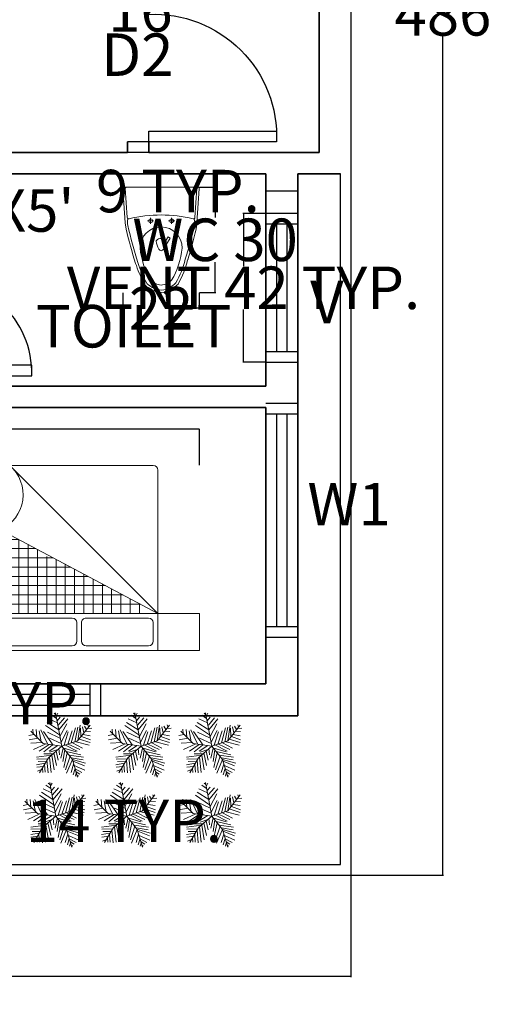
# Model space of a CAD drawing. Units: inches. Extents: x 774 to 1314, y 374 to 930.
# Tile 3 of 5: x 1137 to 1270, y 374 to 652. Entities that reach past the tile are written whole.
import ezdxf
from ezdxf.enums import TextEntityAlignment as Align

# ---------------------------------------------------------------- set-up
doc = ezdxf.new("R2010")
doc.units = ezdxf.units.IN
doc.header["$MEASUREMENT"] = 0
for name, color, linetype, lineweight in [('A-ANNO-DIMS', 2, 'Continuous', 18), ('A-ANNO-TEXT', 2, 'Continuous', 18), ('A-AREA-IDEN', 2, 'Continuous', 18), ('A-DOOR', 6, 'Continuous', 25), ('A-FLOR-FIXT', 9, 'Continuous', 18), ('A-FURN', 8, 'Continuous', 18), ('A-GLAZ', 4, 'Continuous', 18), ('A-WALL', 1, 'Continuous', 35), ('C-PROP', 3, 'Continuous', 25), ('L-PLNT', 3, 'Continuous', 13)]:
    doc.layers.add(name, color=color, linetype=linetype, lineweight=lineweight)
doc.layers.add('Layer4', color=4, linetype='Continuous')
doc.styles.get("Standard").update_dxf_attribs({"font": 'arial.ttf'})
doc.dimstyles.get("Standard").update_dxf_attribs({"dimtxt": 12, "dimasz": 0.18, "dimexe": 0.18, "dimexo": 0.0625, "dimgap": 0.09, "dimtad": 0, "dimtih": 1, "dimtoh": 1, "dimdec": 0, "dimzin": 0, "dimdsep": 46, "dimlunit": 4, "dimtxsty": 'Standard', "dimcen": 0.09, "dimadec": 0, "dimazin": 0, "dimtfac": 1, "dimtdec": 0, "dimtofl": 0, "dimtmove": 0, "dimatfit": 3, "dimfxl": 1, "dimtolj": 1, "dimtzin": 0, "dimarcsym": 0})

# ---------------------------------------------------------------- blocks, each defined once
blk = doc.blocks.new('tr')
at = {"layer": 'Layer4'}
for p, q in [((9, 66), (0, 66)), ((9, 63), (0, 63)), ((0, 63), (0, 3)), ((3, 63), (3, 3)), ((6, 3), (6, 63)), ((9, 3), (9, 63)), ((0, 3), (9, 3)), ((0, 0), (9, 0))]:
    blk.add_line(p, q, dxfattribs=at)
blk = doc.blocks.new('ty')
at = {"layer": 'Layer4'}
for p, q in [((9, 42), (0, 42)), ((9, 39), (0, 39)), ((0, 39), (0, 3)), ((3, 39), (3, 3)), ((6, 3), (6, 39)), ((9, 3), (9, 39)), ((0, 3), (9, 3)), ((0, 0), (9, 0))]:
    blk.add_line(p, q, dxfattribs=at)
blk = doc.blocks.new('A$C4CBC1980')
for p, q in [((0.45, 2), (0, 2)), ((0, 2), (0, 1.6)), ((0, 2), (2.6, 2)), ((2.15, 2), (0.45, 2)), ((0.45, 2), (0.45, 0.05)), ((0.45, 0.05), (0.45, 2)), ((1.225, 1.95), (0.55, 1.95)), ((2.05, 1.95), (1.375, 1.95)), ((2.6, 2), (2.025, 2)), ((2.15, 0.05), (2.15, 2)), ((2.6, 1.6), (2.6, 2)), ((0.5, 1.9), (0.5, 1.7)), ((1.275, 1.7), (1.275, 1.9)), ((1.325, 1.7), (1.325, 1.9)), ((2.1, 1.7), (2.1, 1.9)), ((2.6, 1.6), (0, 1.6)), ((0.45, 1.6), (2.05, 0)), ((0.451, 1.6), (2.15, 0.697)), ((1.225, 1.65), (0.55, 1.65)), ((2.15, 1.6), (0.587, 1.6)), ((0.65, 1.494), (0.65, 1.6)), ((0.75, 1.441), (0.75, 1.6)), ((0.85, 1.388), (0.85, 1.6)), ((0.95, 1.335), (0.95, 1.6)), ((1.05, 1.282), (1.05, 1.6)), ((1.15, 1.229), (1.15, 1.6)), ((1.25, 1.176), (1.25, 1.6)), ((1.35, 1.122), (1.35, 1.6)), ((2.05, 1.65), (1.375, 1.65)), ((1.45, 1.069), (1.45, 1.6)), ((1.55, 1.016), (1.55, 1.6)), ((1.65, 0.986), (1.65, 1.6)), ((1.75, 0.91), (1.75, 1.6)), ((1.85, 0.857), (1.85, 1.6)), ((1.95, 0.804), (1.95, 1.6)), ((2.05, 0.751), (2.05, 1.6)), ((2.15, 1.5), (0.639, 1.5)), ((2.15, 1.4), (0.827, 1.4)), ((2.15, 1.3), (1.016, 1.3)), ((2.15, 1.2), (1.204, 1.2)), ((2.15, 1.1), (1.392, 1.1)), ((2.15, 1), (1.58, 1)), ((2.15, 0.9), (1.769, 0.9)), ((2.15, 0.8), (1.957, 0.8)), ((0.5, 0), (2.1, 0))]:
    blk.add_line(p, q)
for centre, radius, start, end in [((0.55, 1.9), 0.05, 90, 180), ((1.225, 1.9), 0.05, 0, 90), ((1.375, 1.9), 0.05, 90, 180), ((2.05, 1.9), 0.05, 0, 90), ((0.55, 1.7), 0.05, 180, 270), ((1.225, 1.7), 0.05, 270, 0), ((1.375, 1.7), 0.05, 180, 270), ((2.05, 1.7), 0.05, 270, 0), ((2.327, 0.316), 0.421, 114.9633, 228.7161), ((0.5, 0.05), 0.05, 180, 270), ((0.5, 0.05), 0.05, 180, 270), ((2.1, 0.05), 0.05, 270, 0)]:
    blk.add_arc(centre, radius, start, end)
blk = doc.blocks.new('A$C43D762ED')
for p, q in [((0, 0.729), (0.0157, 0.4897)), ((0.5246, 0.7397), (0.01, 0.7397)), ((0.0162, 0.7328), (0.0298, 0.5262)), ((0.5184, 0.7328), (0.5048, 0.5262)), ((0.5346, 0.729), (0.5189, 0.4897)), ((0.0157, 0.4897), (0.0223, 0.4455)), ((0.2151, 0.5034), (0.172, 0.5034)), ((0.1938, 0.525), (0.1938, 0.4814)), ((0.3195, 0.5034), (0.3626, 0.5034)), ((0.3408, 0.525), (0.3408, 0.4814)), ((0.5189, 0.4897), (0.5123, 0.4455)), ((0.2923, 0.3214), (0.3311, 0.382)), ((0.3001, 0.3651), (0.3169, 0.3911)), ((0.3169, 0.3911), (0.3311, 0.382)), ((0.0888, 0.2044), (0.0937, 0.19))]:
    blk.add_line(p, q)
for centre in [(0.1938, 0.5034), (0.3408, 0.5034)]:
    blk.add_circle(centre, 0.0137)
for centre, radius, start, end in [((0.01, 0.7297), 0.01, 90, 183.76235), ((0.0257, 0.7297), 0.01, 90, 161.99285), ((0.5089, 0.7297), 0.01, 18.00715, 90), ((0.5246, 0.7297), 0.01, 356.23765, 90), ((0.0398, 0.5269), 0.01, 183.76235, 283.82831), ((0.1268, 0.4939), 0.0953, 165.17281, 194.54705), ((0.2673, -0.3974), 0.9419, 76.14598, 103.82831), ((0.4948, 0.5269), 0.01, 256.17169, 356.23765), ((0.4078, 0.4939), 0.0953, 345.45295, 14.82719), ((2.7485, 1.0673), 2.7962, 192.84784, 197.97333), ((2.7485, 1.0673), 2.7789, 192.41213, 197.97333), ((0.2675, 0.3121), 0.148, 90, 180), ((0.2675, 0.3121), 0.148, 0, 90), ((-2.2139, 1.0673), 2.7789, 342.53599, 347.58787), ((-2.2139, 1.0673), 2.7962, 342.54844, 347.15216), ((0.2395, 0.3612), 0.006, 139.49966, 184.26121), ((0.3639, 0.3708), 0.1308, 184.40911, 210.02383), ((0.2675, 0.3372), 0.0429, 40.50034, 139.49966), ((0.1712, 0.3708), 0.1308, 329.97617, 355.59089), ((0.2956, 0.3612), 0.006, 355.73879, 40.50034), ((0.6936, 0.3754), 0.5775, 186.28683, 210.10499), ((0.2721, 0.3185), 0.0252, 211.47881, 259.49934), ((0.2629, 0.3185), 0.0252, 280.50066, 328.52119), ((-0.1586, 0.3754), 0.5775, 329.89501, 353.71317), ((0.714, 0.3854), 0.6336, 196.09704, 210.8164), ((-0.1586, 0.3754), 0.6121, 329.89501, 346.57808), ((-0.1586, 0.3754), 0.6294, 329.89501, 346.52221), ((0.7246, 0.3908), 0.662, 197.65406, 211.16701), ((0.2786, 0.1719), 0.1209, 225.50669, 264.71555), ((0.2564, 0.1719), 0.1209, 275.28445, 314.49331), ((0.2834, 0.1859), 0.1862, 227.70774, 266.91661), ((0.2818, 0.1811), 0.1643, 227.04359, 266.25246), ((0.2492, 0.183), 0.1673, 277.51863, 316.7275), ((0.2459, 0.188), 0.1899, 278.30562, 317.51449)]:
    blk.add_arc(centre, radius, start, end)
blk = doc.blocks.new('*U14')
for p, q in [((-8.737, 47.138), (-17.069, 52.711)), ((-10.186, 53.64), (-13.084, 55.962)), ((0, 0), (-10.5, 57)), ((-9.099, 51.782), (-6.563, 55.962)), ((-3.665, 19.273), (-27.574, 35.527)), ((-5.114, 28.097), (-24.676, 40.636)), ((-7.288, 39.707), (-21.778, 46.673)), ((-7.65, 43.423), (-2.578, 49.46)), ((-5.839, 35.992), (4.667, 48.067)), ((-5.114, 27.632), (10.463, 46.673)), ((-2.941, 16.486), (8.652, 37.85)), ((27, 9), (48, 36)), ((27.127, 9.056), (31.112, 35.992)), ((38.719, 34.134), (41.979, 28.561)), ((44.153, 36.456), (45.239, 32.741)), ((-47.498, 19.737), (-55.83, 18.344)), ((-31.5, 4.5), (-52.5, 25.5)), ((-48.585, 21.131), (-49.309, 29.026)), ((-43.513, 28.561), (-42.427, 15.558)), ((-38.442, 26.239), (-34.819, 7.663)), ((-35.544, 28.097), (-24.314, 3.947)), ((-14.533, 2.09), (-30.834, 25.31)), ((-24.314, 23.917), (-2.941, 13.7)), ((-1.129, 6.734), (9.014, 26.704)), ((3.942, 1.625), (11.187, 24.381)), ((10.101, 3.483), (17.708, 26.239)), ((16.259, 5.805), (23.142, 31.348)), ((22.055, 7.198), (27.489, 32.277)), ((31.836, 30.883), (32.561, 16.486)), ((35.096, 32.741), (37.27, 22.524)), ((36.183, 19.737), (48.137, 17.88)), ((40.53, 25.775), (48.862, 24.846)), ((43.791, 29.954), (51.036, 30.883)), ((-40.615, 13.7), (-55.105, 10.913)), ((-33.37, 6.269), (-52.207, 5.34)), ((-28.299, 3.483), (-47.86, -5.805)), ((-21.416, 3.018), (-38.079, -8.128)), ((0, 0), (-31.5, 4.5)), ((-15.982, 2.09), (-30.11, -9.521)), ((0, 0), (-22.5, -19.5)), ((-6.563, 1.161), (-21.416, -8.128)), ((-20.691, 13.7), (-1.129, 4.876)), ((0, 0), (27, 9)), ((0, 0), (18, -22.5)), ((6.478, 1.625), (26.04, -8.592)), ((11.187, 3.483), (30.749, -5.805)), ((18.07, 5.805), (35.096, -3.483)), ((24.229, 7.663), (46.688, 1.625)), ((29.662, 12.307), (48.137, 6.269)), ((33.285, 16.486), (48.862, 10.913)), ((-17.431, -15.094), (-42.789, -18.809)), ((-15.257, -12.772), (-30.11, -12.772)), ((-6.563, -5.805), (-19.967, -9.985)), ((-17.069, -15.094), (-12.721, -40.172)), ((-13.446, -11.378), (-8.737, -32.741)), ((-9.461, -8.592), (-6.201, -23.453)), ((-4.752, -3.483), (-3.665, -14.629)), ((2.493, -3.019), (-1.491, -20.202)), ((1.769, -2.555), (24.229, -9.521)), ((5.029, -6.27), (2.131, -25.775)), ((9.014, -11.378), (3.58, -35.992)), ((7.565, -9.056), (32.198, -14.629)), ((12.274, -15.094), (36.907, -18.809)), ((-28.299, -29.026), (-42.789, -31.348)), ((-24.314, -21.596), (-42.427, -22.06)), ((-26.849, -26.24), (-40.253, -25.775)), ((-22.5, -19.5), (-37.5, -45)), ((-29.023, -30.884), (-27.936, -43.887)), ((-25.038, -23.918), (-22.865, -45.281)), ((-20.691, -18.345), (-17.793, -44.352)), ((14.085, -16.951), (6.478, -40.172)), ((18.07, -22.524), (8.289, -45.745)), ((20.244, -30.419), (15.897, -44.816)), ((16.259, -19.738), (36.183, -22.989)), ((18, -22.5), (27, -52.5)), ((18.433, -22.524), (40.53, -29.026)), ((19.157, -25.311), (38.719, -33.206)), ((21.331, -32.741), (39.081, -40.636)), ((-30.834, -34.135), (-42.427, -35.528)), ((-34.457, -39.708), (-40.978, -42.494)), ((-32.646, -36.921), (-31.921, -44.352)), ((22.78, -37.85), (19.519, -48.532)), ((22.78, -38.314), (34.372, -44.816)), ((24.591, -45.745), (23.142, -50.854)), ((24.591, -43.423), (30.749, -47.603)), ((26.764, -49.925), (28.213, -50.854))]:
    blk.add_line(p, q)
blk = doc.blocks.new('DOOR-SWING-36IN')
blk.add_lwpolyline([(0, 0), (3, 0), (3, 36), (0, 36)], close=True)
blk.add_arc((1.5, 1.5), 34.53, 357.5104, 92.4896)
blk = doc.blocks.new('*D27')
at = {"layer": 'A-ANNO-DIMS', "color": 0, "lineweight": -2, "transparency": 16777216}
for p, q in [((1206.27, 597.38), (1199.85, 597.38)), ((1200.03, 597.2), (1200.03, 582.5)), ((1200.03, 555.56), (1200.03, 570.26)), ((1206.27, 555.38), (1199.85, 555.38))]:
    blk.add_line(p, q, dxfattribs=at)
at = {"layer": 'A-ANNO-DIMS', "color": 0, "transparency": 16777216}
for points in [[(1200, 597.2), (1200.06, 597.2), (1200.03, 597.38)], [(1200, 555.56), (1200.06, 555.56), (1200.03, 555.38)]]:
    blk.add_solid(points, dxfattribs=at)
at = {"layer": 'Defpoints', "color": 0, "transparency": 16777216}
for p in [(1206.33, 597.38), (1200.03, 555.38), (1206.33, 555.38)]:
    blk.add_point(p, dxfattribs=at)
at = {"layer": 'A-ANNO-DIMS', "color": 0, "transparency": 16777216, "insert": (1200.03, 576.38), "char_height": 12, "attachment_point": 5}
blk.add_mtext('\\A1;VENT 42 TYP.', dxfattribs=at)
blk = doc.blocks.new('*D28')
at = {"layer": 'A-ANNO-DIMS', "color": 0, "lineweight": -2, "transparency": 16777216}
for p, q in [((1206.33, 603.68), (1206.15, 603.68)), ((1206.33, 597.44), (1206.33, 603.86)), ((1215.15, 603.68), (1206.51, 603.68)), ((1215.33, 597.44), (1215.33, 603.86))]:
    blk.add_line(p, q, dxfattribs=at)
at = {"layer": 'A-ANNO-DIMS', "color": 0, "transparency": 16777216}
for points in [[(1206.51, 603.71), (1206.51, 603.65), (1206.33, 603.68)], [(1215.15, 603.71), (1215.15, 603.65), (1215.33, 603.68)]]:
    blk.add_solid(points, dxfattribs=at)
at = {"layer": 'Defpoints', "color": 0, "transparency": 16777216}
for p in [(1206.33, 603.68), (1206.33, 597.38), (1215.33, 597.38)]:
    blk.add_point(p, dxfattribs=at)
at = {"layer": 'A-ANNO-DIMS', "color": 0, "transparency": 16777216, "insert": (1181.52, 603.68), "char_height": 12, "attachment_point": 5}
blk.add_mtext('\\A1;9 TYP.', dxfattribs=at)
blk = doc.blocks.new('*D29')
at = {"layer": 'A-ANNO-DIMS', "color": 0, "lineweight": -2, "transparency": 16777216}
for p, q in [((987.33, 464.5), (987.33, 458.92)), ((1023.76, 464.5), (1023.76, 458.92)), ((987.51, 459.1), (1023.58, 459.1)), ((1023.76, 459.1), (1023.94, 459.1))]:
    blk.add_line(p, q, dxfattribs=at)
at = {"layer": 'A-ANNO-DIMS', "color": 0, "transparency": 16777216}
for points in [[(987.51, 459.13), (987.51, 459.07), (987.33, 459.1)], [(1023.58, 459.13), (1023.58, 459.07), (1023.76, 459.1)]]:
    blk.add_solid(points, dxfattribs=at)
at = {"layer": 'Defpoints', "color": 0, "transparency": 16777216}
for p in [(987.33, 464.57), (1023.76, 464.57), (1023.76, 459.1)]:
    blk.add_point(p, dxfattribs=at)
at = {"layer": 'A-ANNO-DIMS', "color": 0, "transparency": 16777216, "insert": (1093.45, 459.1), "char_height": 12, "attachment_point": 5}
blk.add_mtext('\\A1;DOOR D1 36 TYP.', dxfattribs=at)
blk = doc.blocks.new('*D35')
at = {"layer": 'A-ANNO-DIMS', "color": 0, "lineweight": -2, "transparency": 16777216}
for p, q in [((1008.19, 427.87), (1008.19, 425.69)), ((1008.37, 425.87), (1021.76, 425.87)), ((1021.94, 427.87), (1021.94, 425.69)), ((1021.94, 425.87), (1022.12, 425.87))]:
    blk.add_line(p, q, dxfattribs=at)
at = {"layer": 'A-ANNO-DIMS', "color": 0, "transparency": 16777216}
for points in [[(1008.37, 425.9), (1008.37, 425.84), (1008.19, 425.87)], [(1021.76, 425.9), (1021.76, 425.84), (1021.94, 425.87)]]:
    blk.add_solid(points, dxfattribs=at)
at = {"layer": 'Defpoints', "color": 0, "transparency": 16777216}
for p in [(1008.19, 427.93), (1021.94, 427.93), (1021.94, 425.87)]:
    blk.add_point(p, dxfattribs=at)
at = {"layer": 'A-ANNO-DIMS', "color": 0, "transparency": 16777216, "insert": (1112.58, 425.87), "char_height": 12, "attachment_point": 5}
blk.add_mtext('\\A1;ENTRY PAVER 14 TYP.', dxfattribs=at)
blk = doc.blocks.new('*D39')
at = {"layer": 'A-ANNO-DIMS', "color": 0, "lineweight": -2, "transparency": 16777216}
for p, q in [((1119.75, 526.29), (1119.75, 536.6)), ((1187.64, 526.29), (1187.64, 536.6)), ((1119.75, 536.42), (1119.57, 536.42)), ((1187.46, 536.42), (1119.93, 536.42))]:
    blk.add_line(p, q, dxfattribs=at)
at = {"layer": 'A-ANNO-DIMS', "color": 0, "transparency": 16777216}
for points in [[(1119.93, 536.45), (1119.93, 536.39), (1119.75, 536.42)], [(1187.46, 536.45), (1187.46, 536.39), (1187.64, 536.42)]]:
    blk.add_solid(points, dxfattribs=at)
at = {"layer": 'Defpoints', "color": 0, "transparency": 16777216}
for p in [(1119.75, 536.42), (1119.75, 526.23), (1187.64, 526.23)]:
    blk.add_point(p, dxfattribs=at)
at = {"layer": 'A-ANNO-DIMS', "color": 0, "transparency": 16777216, "insert": (1070.98, 536.42), "char_height": 12, "attachment_point": 5}
blk.add_mtext('\\A1;BED 68 TYP.', dxfattribs=at)
blk = doc.blocks.new('*D43')
at = {"layer": 'A-ANNO-DIMS', "color": 0, "lineweight": -2, "transparency": 16777216}
for p, q in [((1187.61, 604.79), (1192.19, 604.79)), ((1192.01, 604.61), (1192.01, 596.22)), ((1192.01, 575.22), (1192.01, 583.62)), ((1187.61, 575.04), (1192.19, 575.04))]:
    blk.add_line(p, q, dxfattribs=at)
at = {"layer": 'A-ANNO-DIMS', "color": 0, "transparency": 16777216}
for points in [[(1191.98, 604.61), (1192.04, 604.61), (1192.01, 604.79)], [(1191.98, 575.22), (1192.04, 575.22), (1192.01, 575.04)]]:
    blk.add_solid(points, dxfattribs=at)
at = {"layer": 'Defpoints', "color": 0, "transparency": 16777216}
for p in [(1187.55, 604.79), (1192.01, 604.79), (1187.55, 575.04)]:
    blk.add_point(p, dxfattribs=at)
at = {"layer": 'A-ANNO-DIMS', "color": 0, "transparency": 16777216, "insert": (1192.01, 589.92), "char_height": 12, "attachment_point": 5}
blk.add_mtext('\\A1;WC 30', dxfattribs=at)
blk = doc.blocks.new('*D44')
at = {"layer": 'A-ANNO-DIMS', "color": 0, "lineweight": -2, "transparency": 16777216}
for p, q in [((1166.04, 574.98), (1166.04, 570.4)), ((1187.55, 574.98), (1187.55, 570.4)), ((1166.22, 570.58), (1168.07, 570.58)), ((1187.37, 570.58), (1185.52, 570.58))]:
    blk.add_line(p, q, dxfattribs=at)
at = {"layer": 'A-ANNO-DIMS', "color": 0, "transparency": 16777216}
for points in [[(1166.22, 570.61), (1166.22, 570.55), (1166.04, 570.58)], [(1187.37, 570.61), (1187.37, 570.55), (1187.55, 570.58)]]:
    blk.add_solid(points, dxfattribs=at)
at = {"layer": 'Defpoints', "color": 0, "transparency": 16777216}
for p in [(1166.04, 575.04), (1187.55, 575.04), (1187.55, 570.58)]:
    blk.add_point(p, dxfattribs=at)
at = {"layer": 'A-ANNO-DIMS', "color": 0, "transparency": 16777216, "insert": (1176.79, 570.58), "char_height": 12, "attachment_point": 5}
blk.add_mtext('\\A1;22', dxfattribs=at)
blk = doc.blocks.new('*D46')
at = {"layer": 'A-ANNO-DIMS', "color": 0, "lineweight": -2, "transparency": 16777216}
for p, q in [((1147.06, 659.75), (1147.06, 654.53)), ((1162.65, 659.75), (1162.65, 654.53)), ((1147.24, 654.71), (1162.47, 654.71)), ((1162.65, 654.71), (1162.83, 654.71))]:
    blk.add_line(p, q, dxfattribs=at)
at = {"layer": 'A-ANNO-DIMS', "color": 0, "transparency": 16777216}
for points in [[(1147.24, 654.74), (1147.24, 654.68), (1147.06, 654.71)], [(1162.47, 654.74), (1162.47, 654.68), (1162.65, 654.71)]]:
    blk.add_solid(points, dxfattribs=at)
at = {"layer": 'Defpoints', "color": 0, "transparency": 16777216}
for p in [(1147.06, 659.82), (1162.65, 659.82), (1162.65, 654.71)]:
    blk.add_point(p, dxfattribs=at)
at = {"layer": 'A-ANNO-DIMS', "color": 0, "transparency": 16777216, "insert": (1170.95, 654.71), "char_height": 12, "attachment_point": 5}
blk.add_mtext('\\A1;16', dxfattribs=at)
blk = doc.blocks.new('*D53')
at = {"layer": 'A-ANNO-DIMS', "color": 0, "lineweight": -2, "transparency": 16777216}
for p, q in [((864.33, 410.5), (864.33, 381.78)), ((1230.33, 410.5), (1230.33, 381.78)), ((864.51, 381.96), (1034, 381.96)), ((1230.15, 381.96), (1060.67, 381.96))]:
    blk.add_line(p, q, dxfattribs=at)
at = {"layer": 'A-ANNO-DIMS', "color": 0, "transparency": 16777216}
for points in [[(864.51, 381.99), (864.51, 381.93), (864.33, 381.96)], [(1230.15, 381.99), (1230.15, 381.93), (1230.33, 381.96)]]:
    blk.add_solid(points, dxfattribs=at)
at = {"layer": 'Defpoints', "color": 0, "transparency": 16777216}
for p in [(864.33, 410.57), (1230.33, 410.57), (1230.33, 381.96)]:
    blk.add_point(p, dxfattribs=at)
at = {"layer": 'A-ANNO-DIMS', "color": 0, "transparency": 16777216, "insert": (1047.33, 381.96), "char_height": 12, "attachment_point": 5}
blk.add_mtext('\\A1;366', dxfattribs=at)
blk = doc.blocks.new('*D54')
at = {"layer": 'A-ANNO-DIMS', "color": 0, "lineweight": -2, "transparency": 16777216}
for p, q in [((1230.4, 896.57), (1256.44, 896.57)), ((1256.26, 896.39), (1256.26, 659.78)), ((1256.26, 410.75), (1256.26, 647.35)), ((1230.4, 410.57), (1256.44, 410.57))]:
    blk.add_line(p, q, dxfattribs=at)
at = {"layer": 'A-ANNO-DIMS', "color": 0, "transparency": 16777216}
for points in [[(1256.23, 896.39), (1256.29, 896.39), (1256.26, 896.57)], [(1256.23, 410.75), (1256.29, 410.75), (1256.26, 410.57)]]:
    blk.add_solid(points, dxfattribs=at)
at = {"layer": 'Defpoints', "color": 0, "transparency": 16777216}
for p in [(1230.33, 896.57), (1256.26, 896.57), (1230.33, 410.57)]:
    blk.add_point(p, dxfattribs=at)
at = {"layer": 'A-ANNO-DIMS', "color": 0, "transparency": 16777216, "insert": (1256.26, 653.57), "char_height": 12, "attachment_point": 5}
blk.add_mtext('\\A1;486', dxfattribs=at)

msp = doc.modelspace()

# ---------------------------------------------------------------- linework, layer by layer
at = {"layer": 'A-DOOR'}
for p, q in [((1173.3347, 617.5656), (1167.3347, 617.5656)), ((1173.3347, 614.5656), (1167.3347, 614.5656))]:
    msp.add_line(p, q, dxfattribs=at)
msp.add_lwpolyline([(1110.3347, 551.5656), (1140.3347, 551.5656), (1140.3347, 554.5656), (1110.3347, 554.5656)], close=True, dxfattribs=at)
msp.add_arc((1113.8597, 552.3156), 26.4856, 358.377324, 97.648251, dxfattribs=at)
at = {"layer": 'A-WALL'}
for p, q in [((1167.3347, 614.5656), (1065.3347, 614.5656)), ((1167.3347, 614.5656), (1146.3347, 614.5656)), ((1221.3347, 614.5656), (1173.3347, 614.5656)), ((1206.3347, 608.5656), (1110.3347, 608.5656)), ((1206.3347, 608.5656), (1203.3347, 608.5656)), ((1206.3347, 548.5656), (1206.3347, 608.5656)), ((1206.3347, 548.5656), (1206.3347, 608.5656)), ((1227.3347, 608.5656), (1215.3347, 608.5656)), ((1206.3347, 548.5656), (1110.3347, 548.5656)), ((1206.3347, 542.5656), (1104.3347, 542.5656)), ((1206.3347, 464.5656), (1206.3347, 542.5656)), ((1206.3347, 464.5656), (1065.3347, 464.5656)), ((1215.3347, 455.5656), (1023.3347, 455.5656))]:
    msp.add_line(p, q, dxfattribs=at)
for points in [[(1221.3347, 614.5656), (1221.3347, 734.5656)], [(1167.3347, 614.5656), (1167.3347, 617.5656)], [(1173.3347, 614.5656), (1173.3347, 617.5656)], [(1215.3347, 455.5656), (1215.3347, 608.5656)]]:
    msp.add_lwpolyline(points, dxfattribs=at)
at = {"layer": 'C-PROP'}
msp.add_lwpolyline([(864.3347, 410.5656), (1230.3347, 410.5656), (1230.3347, 896.5656), (864.3347, 896.5656)], close=True, dxfattribs=at)
for points in [[(1194.3347, 413.5656), (1227.3347, 413.5656), (1227.3347, 608.5656)], [(984.3347, 413.5656), (1194.3347, 413.5656)]]:
    msp.add_lwpolyline(points, dxfattribs=at)

# ---------------------------------------------------------------- block references
at = {"layer": 'A-DOOR', "extrusion": (0, 0, -1), "zscale": -1, "rotation": 89.9999999999994}
msp.add_blockref('DOOR-SWING-36IN', (-1173.3351, 617.5659), dxfattribs=at)
at = {"layer": 'A-FLOR-FIXT', "xscale": 40.21700905222547, "yscale": 40.21700905222547, "zscale": 40.21700905222547}
msp.add_blockref('A$C43D762ED', (1166.0432, 575.0431), dxfattribs=at)
at = {"layer": 'A-FURN', "xscale": 26.11182411513011, "yscale": 26.11182411513011, "zscale": 26.11182411513011, "rotation": 180}
msp.add_blockref('A$C4CBC1980', (1187.6404, 526.2325), dxfattribs=at)
at = {"layer": 'A-GLAZ'}
for name, p, rotation in [('ty', (1215.3347, 597.3811), 180), ('tr', (1093.8347, 464.5656), 270)]:
    msp.add_blockref(name, p, dxfattribs=dict(at, rotation=rotation))
msp.add_blockref('tr', (1206.3347, 477.741), dxfattribs=at)
at = {"layer": 'L-PLNT', "xscale": 0.1661250524681751, "yscale": 0.1661250524681751, "zscale": 0.1661250524681751}
for p in [(1148.7719, 446.9445), (1171.149, 446.9445), (1191.0841, 446.9445), (1147.129, 427.2022), (1167.0862, 427.2022), (1191.0776, 427.2022)]:
    msp.add_blockref('*U14', p, dxfattribs=at)

# ---------------------------------------------------------------- texts
at = {"layer": 'A-ANNO-TEXT'}
for s, p in [('D2', (1170.092, 636.1816)), ('V', (1223.5388, 566.3684)), ('W1', (1229.7763, 509.2862))]:
    msp.add_text(s, height=12, dxfattribs=at).set_placement(p, align=Align.CENTER)
at = {"layer": 'A-AREA-IDEN'}
for s, p in [("8'X5'", (1134.0548, 592.198)), ('TOILET', (1169.0599, 559.5219))]:
    msp.add_text(s, height=12, dxfattribs=at).set_placement(p, align=Align.CENTER)

# ---------------------------------------------------------------- dimensions: what is measured, and where the dimension line sits
at = {"layer": 'A-ANNO-DIMS'}
dim = msp.add_linear_dim(base=(1256.2597, 896.5656), p1=(1230.3347, 410.5656), p2=(1230.3347, 896.5656), angle=90, dimstyle='Standard', override={"dimdec": 0, "dimlfac": 1, "dimrnd": 0, "dimzin": 0, "dimdsep": 46, "dimlunit": 2}, dxfattribs=at)
dim.commit()
dim.dimension.update_dxf_attribs({"geometry": '*D54', "text_midpoint": (1256.2597, 653.5656)})
for base, p1, p2, picture, middle in [((1162.654, 654.7071), (1147.065, 659.8154), (1162.654, 659.8154), '*D46', (1170.9499, 654.7071)), ((1187.5504, 570.5809), (1166.0359, 575.0431), (1187.5504, 575.0431), '*D44', (1176.7932, 570.5809)), ((1230.3347, 381.9636), (864.3347, 410.5656), (1230.3347, 410.5656), '*D53', (1047.3347, 381.9636))]:
    dim = msp.add_linear_dim(base=base, p1=p1, p2=p2, dimstyle='Standard', override={"dimdec": 0, "dimlfac": 1, "dimrnd": 0, "dimzin": 0, "dimdsep": 46, "dimlunit": 2}, dxfattribs=at)
    dim.commit()
    dim.dimension.update_dxf_attribs({"geometry": picture, "text_midpoint": middle})
for base, p1, p2, angle, text, picture, middle in [((1206.3347, 603.6811), (1215.3347, 597.3811), (1206.3347, 597.3811), 180, '<> TYP.', '*D28', (1181.5204, 603.6811)), ((1192.0126, 604.7911), (1187.5504, 575.0431), (1187.5504, 604.7911), 90, 'WC <>', '*D43', (1192.0126, 589.9171)), ((1200.0347, 555.3811), (1206.3347, 597.3811), (1206.3347, 555.3811), 270, 'VENT <> TYP.', '*D27', (1200.0347, 576.3811)), ((1119.75, 536.4161), (1187.6407, 526.2324), (1119.75, 526.2324), 180, 'BED <> TYP.', '*D39', (1070.9766, 536.4161))]:
    dim = msp.add_linear_dim(base=base, p1=p1, p2=p2, angle=angle, text=text, dimstyle='Standard', override={"dimdec": 0, "dimlfac": 1, "dimrnd": 0, "dimzin": 0, "dimdsep": 46, "dimlunit": 2}, dxfattribs=at)
    dim.commit()
    dim.dimension.update_dxf_attribs({"geometry": picture, "text_midpoint": middle})
for base, p1, p2, text, picture, middle in [((1023.7552, 459.1025), (987.3347, 464.5656), (1023.7552, 464.5656), 'DOOR D1 <> TYP.', '*D29', (1093.4508, 459.1025)), ((1021.9366, 425.8667), (1008.1858, 427.9294), (1021.9366, 427.9294), 'ENTRY PAVER <> TYP.', '*D35', (1112.5791, 425.8667))]:
    dim = msp.add_linear_dim(base=base, p1=p1, p2=p2, text=text, dimstyle='Standard', override={"dimdec": 0, "dimlfac": 1, "dimrnd": 0, "dimzin": 0, "dimdsep": 46, "dimlunit": 2}, dxfattribs=at)
    dim.commit()
    dim.dimension.update_dxf_attribs({"geometry": picture, "text_midpoint": middle})

doc.saveas('drawing.dxf')
